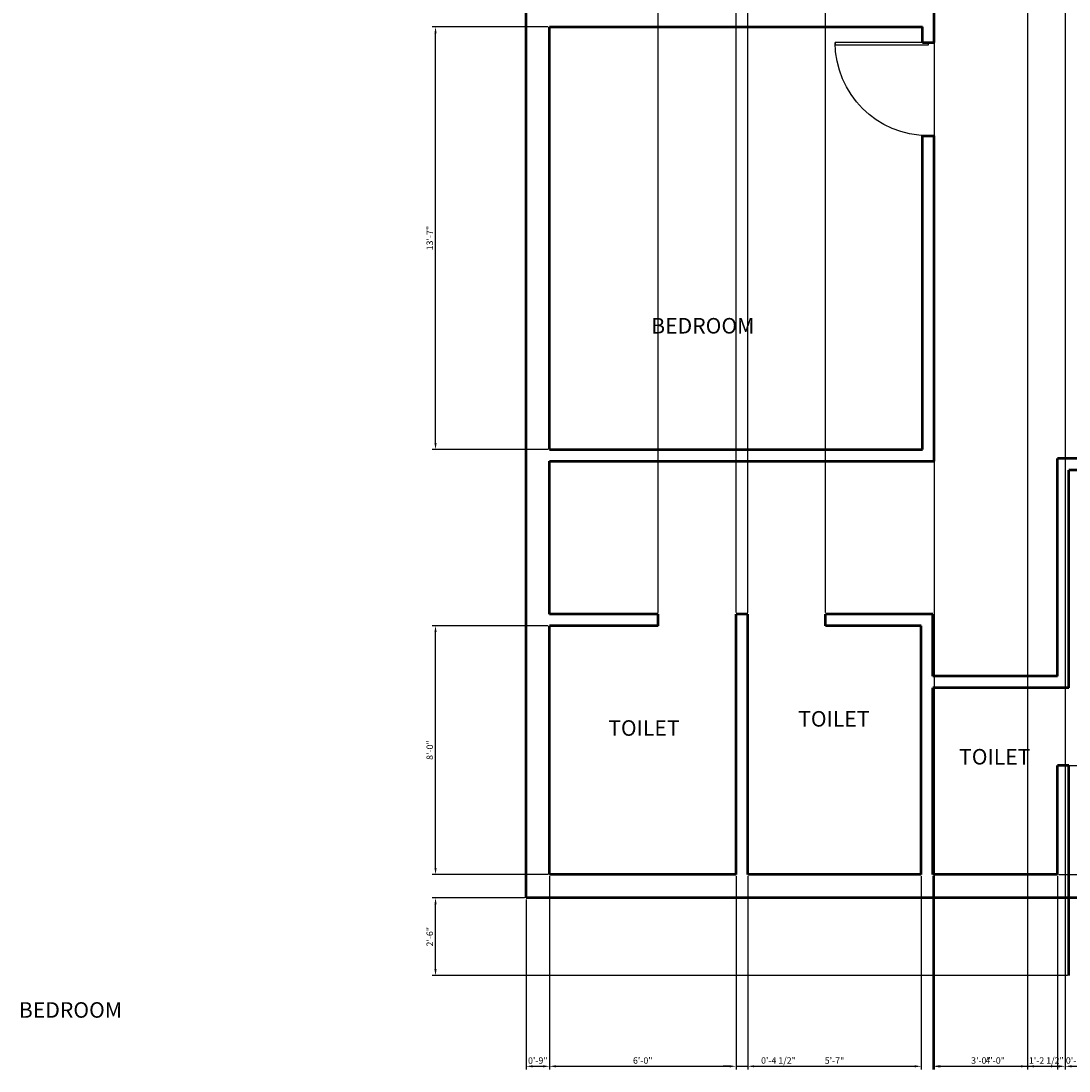
# Model space of a CAD drawing. Units: inches. Extents: x 877 to 2164, y 771 to 1603.
# Tile 1 of 6: x 877 to 1281, y 771 to 1176. Entities that reach past the tile are written whole.
import ezdxf

# ---------------------------------------------------------------- set-up
doc = ezdxf.new("R2010")
doc.units = ezdxf.units.IN
for name, color, linetype, lineweight in [('A-ANNO-DIMS', 2, 'Continuous', 18), ('A-AREA-IDEN', 7, 'Continuous', 25), ('A-DOOR', 5, 'Continuous', 25), ('A-WALL', 7, 'Continuous', 50)]:
    doc.layers.add(name, color=color, linetype=linetype, lineweight=lineweight)
doc.styles.get("Standard").update_dxf_attribs({"font": 'arial.ttf'})
doc.dimstyles.new('ISO-25', dxfattribs={"dimtxt": 2.5, "dimasz": 2.5, "dimexe": 1.25, "dimexo": 0.625, "dimtad": 1, "dimdec": 0, "dimlunit": 4, "dimtxsty": 'Standard', "dimcen": 2.5, "dimadec": 0, "dimazin": 0, "dimtfac": 1, "dimtdec": 0, "dimtmove": 0, "dimatfit": 3, "dimfxl": 1, "dimarcsym": 0})

# ---------------------------------------------------------------- blocks, each defined once
blk = doc.blocks.new('DOOR-SINGLE-36IN')
blk.add_lwpolyline([(0, 0), (0, 1), (36, 1), (36, 0)], close=True)
blk.add_arc((36, 0), 36, 90, 180)
blk = doc.blocks.new('*D16')
at = {"layer": 'A-ANNO-DIMS', "color": 0, "lineweight": -2, "transparency": 16777216}
for p, q in [((1080.27, 1173.62), (1035.67, 1173.62)), ((1036.92, 1013.12), (1036.92, 1171.12)), ((1080.27, 1010.62), (1035.67, 1010.62))]:
    blk.add_line(p, q, dxfattribs=at)
at = {"layer": 'A-ANNO-DIMS', "color": 0, "transparency": 16777216}
for points in [[(1036.5, 1171.12), (1037.34, 1171.12), (1036.92, 1173.62)], [(1036.5, 1013.12), (1037.34, 1013.12), (1036.92, 1010.62)]]:
    blk.add_solid(points, dxfattribs=at)
at = {"layer": 'Defpoints', "color": 0, "transparency": 16777216}
for p in [(1036.92, 1173.62), (1080.89, 1173.62), (1080.89, 1010.62)]:
    blk.add_point(p, dxfattribs=at)
at = {"layer": 'A-ANNO-DIMS', "color": 0, "transparency": 16777216, "insert": (1035.02, 1092.12), "char_height": 2.5, "attachment_point": 5, "rotation": 90}
blk.add_mtext('13\'-7"', dxfattribs=at)
blk = doc.blocks.new('*D24')
at = {"layer": 'A-ANNO-DIMS', "color": 0, "lineweight": -2, "transparency": 16777216}
for p, q in [((1080.89, 846), (1080.89, 771.4)), ((1152.89, 846), (1152.89, 771.4)), ((1083.39, 772.65), (1150.39, 772.65))]:
    blk.add_line(p, q, dxfattribs=at)
at = {"layer": 'A-ANNO-DIMS', "color": 0, "transparency": 16777216}
for points in [[(1083.39, 773.06), (1083.39, 772.23), (1080.89, 772.65)], [(1150.39, 773.06), (1150.39, 772.23), (1152.89, 772.65)]]:
    blk.add_solid(points, dxfattribs=at)
at = {"layer": 'Defpoints', "color": 0, "transparency": 16777216}
for p in [(1080.89, 846.62), (1152.89, 846.62), (1152.89, 772.65)]:
    blk.add_point(p, dxfattribs=at)
at = {"layer": 'A-ANNO-DIMS', "color": 0, "transparency": 16777216, "insert": (1116.89, 774.55), "char_height": 2.5, "attachment_point": 5}
blk.add_mtext('6\'-0"', dxfattribs=at)
blk = doc.blocks.new('*D25')
at = {"layer": 'A-ANNO-DIMS', "color": 0, "lineweight": -2, "transparency": 16777216}
for p, q in [((1157.39, 846), (1157.39, 771.4)), ((1224.39, 846), (1224.39, 771.4)), ((1159.89, 772.65), (1221.89, 772.65))]:
    blk.add_line(p, q, dxfattribs=at)
at = {"layer": 'A-ANNO-DIMS', "color": 0, "transparency": 16777216}
for points in [[(1159.89, 773.06), (1159.89, 772.23), (1157.39, 772.65)], [(1221.89, 773.06), (1221.89, 772.23), (1224.39, 772.65)]]:
    blk.add_solid(points, dxfattribs=at)
at = {"layer": 'Defpoints', "color": 0, "transparency": 16777216}
for p in [(1157.39, 846.62), (1224.39, 846.62), (1224.39, 772.65)]:
    blk.add_point(p, dxfattribs=at)
at = {"layer": 'A-ANNO-DIMS', "color": 0, "transparency": 16777216, "insert": (1190.89, 774.54), "char_height": 2.5, "attachment_point": 5}
blk.add_mtext('5\'-7"', dxfattribs=at)
blk = doc.blocks.new('*D26')
at = {"layer": 'A-ANNO-DIMS', "color": 0, "lineweight": -2, "transparency": 16777216}
for p, q in [((1228.89, 846), (1228.89, 771.4)), ((1276.89, 846), (1276.89, 771.4)), ((1231.39, 772.65), (1274.39, 772.65))]:
    blk.add_line(p, q, dxfattribs=at)
at = {"layer": 'A-ANNO-DIMS', "color": 0, "transparency": 16777216}
for points in [[(1231.39, 773.06), (1231.39, 772.23), (1228.89, 772.65)], [(1274.39, 773.06), (1274.39, 772.23), (1276.89, 772.65)]]:
    blk.add_solid(points, dxfattribs=at)
at = {"layer": 'Defpoints', "color": 0, "transparency": 16777216}
for p in [(1228.89, 846.62), (1276.89, 846.62), (1276.89, 772.65)]:
    blk.add_point(p, dxfattribs=at)
at = {"layer": 'A-ANNO-DIMS', "color": 0, "transparency": 16777216, "insert": (1252.89, 774.55), "char_height": 2.5, "attachment_point": 5}
blk.add_mtext('4\'-0"', dxfattribs=at)
blk = doc.blocks.new('*D28')
at = {"layer": 'A-ANNO-DIMS', "color": 0, "lineweight": -2, "transparency": 16777216}
for p, q in [((1080.27, 942.62), (1035.67, 942.62)), ((1036.92, 849.12), (1036.92, 940.12)), ((1080.27, 846.62), (1035.67, 846.62))]:
    blk.add_line(p, q, dxfattribs=at)
at = {"layer": 'A-ANNO-DIMS', "color": 0, "transparency": 16777216}
for points in [[(1036.5, 940.12), (1037.34, 940.12), (1036.92, 942.62)], [(1036.5, 849.12), (1037.34, 849.12), (1036.92, 846.62)]]:
    blk.add_solid(points, dxfattribs=at)
at = {"layer": 'Defpoints', "color": 0, "transparency": 16777216}
for p in [(1036.92, 942.62), (1080.89, 942.62), (1080.89, 846.62)]:
    blk.add_point(p, dxfattribs=at)
at = {"layer": 'A-ANNO-DIMS', "color": 0, "transparency": 16777216, "insert": (1035.02, 894.62), "char_height": 2.5, "attachment_point": 5, "rotation": 90}
blk.add_mtext('8\'-0"', dxfattribs=at)
blk = doc.blocks.new('*D29')
at = {"layer": 'A-ANNO-DIMS', "color": 0, "lineweight": -2, "transparency": 16777216}
for p, q in [((1277.52, 888.62), (1708.12, 888.62)), ((1706.87, 849.12), (1706.87, 886.12)), ((1277.52, 846.62), (1708.12, 846.62))]:
    blk.add_line(p, q, dxfattribs=at)
at = {"layer": 'A-ANNO-DIMS', "color": 0, "transparency": 16777216}
for points in [[(1706.45, 886.12), (1707.29, 886.12), (1706.87, 888.62)], [(1706.45, 849.12), (1707.29, 849.12), (1706.87, 846.62)]]:
    blk.add_solid(points, dxfattribs=at)
at = {"layer": 'Defpoints', "color": 0, "transparency": 16777216}
for p in [(1276.89, 888.62), (1706.87, 888.62), (1276.89, 846.62)]:
    blk.add_point(p, dxfattribs=at)
at = {"layer": 'A-ANNO-DIMS', "color": 0, "transparency": 16777216, "insert": (1704.97, 867.62), "char_height": 2.5, "attachment_point": 5, "rotation": 90}
blk.add_mtext('3\'-6"', dxfattribs=at)
blk = doc.blocks.new('*D31')
at = {"layer": 'A-ANNO-DIMS', "color": 0, "lineweight": -2, "transparency": 16777216}
for p, q in [((1071.27, 837.62), (1035.67, 837.62)), ((1036.92, 810.12), (1036.92, 835.12)), ((1280.77, 807.62), (1035.67, 807.62))]:
    blk.add_line(p, q, dxfattribs=at)
at = {"layer": 'A-ANNO-DIMS', "color": 0, "transparency": 16777216}
for points in [[(1036.5, 835.12), (1037.34, 835.12), (1036.92, 837.62)], [(1036.5, 810.12), (1037.34, 810.12), (1036.92, 807.62)]]:
    blk.add_solid(points, dxfattribs=at)
at = {"layer": 'Defpoints', "color": 0, "transparency": 16777216}
for p in [(1036.92, 837.62), (1071.89, 837.62), (1281.39, 807.62)]:
    blk.add_point(p, dxfattribs=at)
at = {"layer": 'A-ANNO-DIMS', "color": 0, "transparency": 16777216, "insert": (1035.02, 822.62), "char_height": 2.5, "attachment_point": 5, "rotation": 90}
blk.add_mtext('2\'-6"', dxfattribs=at)
blk = doc.blocks.new('*D32')
at = {"layer": 'A-ANNO-DIMS', "color": 0, "lineweight": -2, "transparency": 16777216}
for p, q in [((1080.89, 846), (1080.89, 771.4)), ((1071.89, 837), (1071.89, 771.4)), ((1074.39, 772.65), (1078.39, 772.65))]:
    blk.add_line(p, q, dxfattribs=at)
at = {"layer": 'A-ANNO-DIMS', "color": 0, "transparency": 16777216}
for points in [[(1074.39, 773.06), (1074.39, 772.23), (1071.89, 772.65)], [(1078.39, 773.06), (1078.39, 772.23), (1080.89, 772.65)]]:
    blk.add_solid(points, dxfattribs=at)
at = {"layer": 'Defpoints', "color": 0, "transparency": 16777216}
for p in [(1080.89, 846.62), (1071.89, 837.62), (1080.89, 772.65)]:
    blk.add_point(p, dxfattribs=at)
at = {"layer": 'A-ANNO-DIMS', "color": 0, "transparency": 16777216, "insert": (1076.39, 774.55), "char_height": 2.5, "attachment_point": 5}
blk.add_mtext('0\'-9"', dxfattribs=at)
blk = doc.blocks.new('*D33')
at = {"layer": 'A-ANNO-DIMS', "color": 0, "lineweight": -2, "transparency": 16777216}
for p, q in [((1152.89, 846), (1152.89, 771.4)), ((1157.39, 846), (1157.39, 771.4)), ((1150.39, 772.65), (1147.89, 772.65)), ((1152.89, 772.65), (1157.39, 772.65)), ((1159.89, 772.65), (1176.12, 772.65))]:
    blk.add_line(p, q, dxfattribs=at)
at = {"layer": 'A-ANNO-DIMS', "color": 0, "transparency": 16777216}
for points in [[(1150.39, 773.06), (1150.39, 772.23), (1152.89, 772.65)], [(1159.89, 773.06), (1159.89, 772.23), (1157.39, 772.65)]]:
    blk.add_solid(points, dxfattribs=at)
at = {"layer": 'Defpoints', "color": 0, "transparency": 16777216}
for p in [(1152.89, 846.62), (1157.39, 846.62), (1157.39, 772.65)]:
    blk.add_point(p, dxfattribs=at)
at = {"layer": 'A-ANNO-DIMS', "color": 0, "transparency": 16777216, "insert": (1169.26, 774.56), "char_height": 2.5, "attachment_point": 5}
blk.add_mtext('0\'-4 1/2"', dxfattribs=at)
blk = doc.blocks.new('*D34')
at = {"layer": 'A-ANNO-DIMS', "color": 0, "lineweight": -2, "transparency": 16777216}
for p, q in [((1122.89, 947.75), (1122.89, 1533.85)), ((1125.39, 1532.6), (1150.39, 1532.6)), ((1152.89, 947.75), (1152.89, 1533.85))]:
    blk.add_line(p, q, dxfattribs=at)
at = {"layer": 'A-ANNO-DIMS', "color": 0, "transparency": 16777216}
for points in [[(1125.39, 1533.01), (1125.39, 1532.18), (1122.89, 1532.6)], [(1150.39, 1533.01), (1150.39, 1532.18), (1152.89, 1532.6)]]:
    blk.add_solid(points, dxfattribs=at)
at = {"layer": 'Defpoints', "color": 0, "transparency": 16777216}
for p in [(1152.89, 1532.6), (1122.89, 947.12), (1152.89, 947.12)]:
    blk.add_point(p, dxfattribs=at)
at = {"layer": 'A-ANNO-DIMS', "color": 0, "transparency": 16777216, "insert": (1137.89, 1534.5), "char_height": 2.5, "attachment_point": 5}
blk.add_mtext('2\'-6"', dxfattribs=at)
blk = doc.blocks.new('*D35')
at = {"layer": 'A-ANNO-DIMS', "color": 0, "lineweight": -2, "transparency": 16777216}
for p, q in [((1157.39, 947.75), (1157.39, 1533.85)), ((1159.89, 1532.6), (1184.89, 1532.6)), ((1187.39, 947.75), (1187.39, 1533.85))]:
    blk.add_line(p, q, dxfattribs=at)
at = {"layer": 'A-ANNO-DIMS', "color": 0, "transparency": 16777216}
for points in [[(1159.89, 1533.01), (1159.89, 1532.18), (1157.39, 1532.6)], [(1184.89, 1533.01), (1184.89, 1532.18), (1187.39, 1532.6)]]:
    blk.add_solid(points, dxfattribs=at)
at = {"layer": 'Defpoints', "color": 0, "transparency": 16777216}
for p in [(1187.39, 1532.6), (1157.39, 947.12), (1187.39, 947.12)]:
    blk.add_point(p, dxfattribs=at)
at = {"layer": 'A-ANNO-DIMS', "color": 0, "transparency": 16777216, "insert": (1172.39, 1534.5), "char_height": 2.5, "attachment_point": 5}
blk.add_mtext('2\'-6"', dxfattribs=at)
blk = doc.blocks.new('*D37')
at = {"layer": 'A-ANNO-DIMS', "color": 0, "lineweight": -2, "transparency": 16777216}
for p, q in [((1229.39, 1392), (1229.39, 771.4)), ((1265.39, 1392), (1265.39, 771.4)), ((1231.89, 772.65), (1262.89, 772.65))]:
    blk.add_line(p, q, dxfattribs=at)
at = {"layer": 'A-ANNO-DIMS', "color": 0, "transparency": 16777216}
for points in [[(1231.89, 773.06), (1231.89, 772.23), (1229.39, 772.65)], [(1262.89, 773.06), (1262.89, 772.23), (1265.39, 772.65)]]:
    blk.add_solid(points, dxfattribs=at)
at = {"layer": 'Defpoints', "color": 0, "transparency": 16777216}
for p in [(1229.39, 1392.62), (1265.39, 1392.62), (1265.39, 772.65)]:
    blk.add_point(p, dxfattribs=at)
at = {"layer": 'A-ANNO-DIMS', "color": 0, "transparency": 16777216, "insert": (1247.39, 774.55), "char_height": 2.5, "attachment_point": 5}
blk.add_mtext('3\'-0"', dxfattribs=at)
blk = doc.blocks.new('*D43')
at = {"layer": 'A-ANNO-DIMS', "color": 0, "lineweight": -2, "transparency": 16777216}
for p, q in [((1279.89, 1452), (1279.89, 771.4)), ((1265.39, 1442), (1265.39, 771.4)), ((1267.89, 772.65), (1277.39, 772.65))]:
    blk.add_line(p, q, dxfattribs=at)
at = {"layer": 'A-ANNO-DIMS', "color": 0, "transparency": 16777216}
for points in [[(1267.89, 773.06), (1267.89, 772.23), (1265.39, 772.65)], [(1277.39, 773.06), (1277.39, 772.23), (1279.89, 772.65)]]:
    blk.add_solid(points, dxfattribs=at)
at = {"layer": 'Defpoints', "color": 0, "transparency": 16777216}
for p in [(1279.89, 1452.62), (1265.39, 1442.62), (1279.89, 772.65)]:
    blk.add_point(p, dxfattribs=at)
at = {"layer": 'A-ANNO-DIMS', "color": 0, "transparency": 16777216, "insert": (1272.64, 774.56), "char_height": 2.5, "attachment_point": 5}
blk.add_mtext('1\'-2 1/2"', dxfattribs=at)
blk = doc.blocks.new('*D44')
at = {"layer": 'A-ANNO-DIMS', "color": 0, "lineweight": -2, "transparency": 16777216}
for p, q in [((1279.89, 1452), (1279.89, 771.4)), ((1289.89, 1452), (1289.89, 771.4)), ((1282.39, 772.65), (1287.39, 772.65))]:
    blk.add_line(p, q, dxfattribs=at)
at = {"layer": 'A-ANNO-DIMS', "color": 0, "transparency": 16777216}
for points in [[(1282.39, 773.06), (1282.39, 772.23), (1279.89, 772.65)], [(1287.39, 773.06), (1287.39, 772.23), (1289.89, 772.65)]]:
    blk.add_solid(points, dxfattribs=at)
at = {"layer": 'Defpoints', "color": 0, "transparency": 16777216}
for p in [(1279.89, 1452.62), (1289.89, 1452.62), (1289.89, 772.65)]:
    blk.add_point(p, dxfattribs=at)
at = {"layer": 'A-ANNO-DIMS', "color": 0, "transparency": 16777216, "insert": (1284.89, 774.55), "char_height": 2.5, "attachment_point": 5}
blk.add_mtext('0\'-10"', dxfattribs=at)

msp = doc.modelspace()

# ---------------------------------------------------------------- linework, layer by layer
at = {"layer": 'A-WALL'}
for p, q in [((1071.89, 837.62), (1071.89, 1497.62)), ((1229.39, 1167.62), (1229.39, 1298.12)), ((1080.89, 1173.62), (1224.89, 1173.62)), ((1080.89, 1010.62), (1080.89, 1173.62)), ((1224.89, 1167.62), (1224.89, 1173.62)), ((1224.89, 1167.62), (1229.39, 1167.62)), ((1224.89, 1010.62), (1224.89, 1131.62)), ((1224.89, 1131.62), (1229.39, 1131.62)), ((1229.39, 1006.12), (1229.39, 1131.62)), ((1080.89, 1010.62), (1224.89, 1010.62)), ((1080.89, 1006.12), (1229.39, 1006.12)), ((1080.89, 947.12), (1080.89, 1006.12)), ((1276.89, 923.12), (1276.89, 1007.12)), ((1373.89, 1007.12), (1276.89, 1007.12)), ((1281.39, 918.62), (1281.39, 1002.62)), ((1373.89, 1002.62), (1281.39, 1002.62)), ((1122.89, 947.12), (1080.89, 947.12)), ((1122.89, 942.62), (1122.89, 947.12)), ((1152.89, 846.62), (1152.89, 947.12)), ((1157.39, 947.12), (1152.89, 947.12)), ((1157.39, 846.62), (1157.39, 947.12)), ((1228.89, 947.12), (1187.39, 947.12)), ((1187.39, 942.62), (1187.39, 947.12)), ((1228.89, 923.12), (1228.89, 947.12)), ((1080.89, 846.62), (1080.89, 942.62)), ((1122.89, 942.62), (1080.89, 942.62)), ((1224.39, 942.62), (1187.39, 942.62)), ((1224.39, 846.62), (1224.39, 942.62)), ((1276.89, 923.12), (1228.89, 923.12)), ((1228.89, 846.62), (1228.89, 918.62)), ((1281.39, 918.62), (1228.89, 918.62)), ((1276.89, 846.62), (1276.89, 888.62)), ((1281.39, 888.62), (1276.89, 888.62)), ((1281.39, 807.62), (1281.39, 888.62)), ((1152.89, 846.62), (1080.89, 846.62)), ((1224.39, 846.62), (1157.39, 846.62)), ((1276.89, 846.62), (1228.89, 846.62)), ((1671.89, 837.62), (1071.89, 837.62))]:
    msp.add_line(p, q, dxfattribs=at)

# ---------------------------------------------------------------- block references
at = {"layer": 'A-DOOR', "extrusion": (0, 0, -1), "zscale": -1, "rotation": 180}
msp.add_blockref('DOOR-SINGLE-36IN', (-1191.15, 1167.62), dxfattribs=at)

# ---------------------------------------------------------------- texts
at = {"layer": 'A-AREA-IDEN', "char_height": 6, "attachment_point": 1}
for s, width, insert in [('BEDROOM', 54.8109, (1120.14, 1061.31)), ('TOILET', 34.9534, (1176.87, 909.68)), ('TOILET', 34.9534, (1103.56, 906.14)), ('TOILET', 34.9534, (1238.97, 895.05)), ('BEDROOM', 54.8109, (876.12, 797.38))]:
    msp.add_mtext_dynamic_manual_height_columns(s, width=width, gutter_width=12.5, heights=[0], dxfattribs=dict(at, insert=insert))

# ---------------------------------------------------------------- dimensions: what is measured, and where the dimension line sits
at = {"layer": 'A-ANNO-DIMS'}
for base, p1, p2, picture, middle in [((1152.89, 1532.6), (1122.89, 947.12), (1152.89, 947.12), '*D34', (1137.89, 1534.5)), ((1187.39, 1532.6), (1157.39, 947.12), (1187.39, 947.12), '*D35', (1172.39, 1534.5)), ((1279.89, 772.65), (1265.39, 1442.62), (1279.89, 1452.62), '*D43', (1272.64, 774.56)), ((1289.89, 772.65), (1279.89, 1452.62), (1289.89, 1452.62), '*D44', (1284.89, 774.55)), ((1265.39, 772.65), (1229.39, 1392.62), (1265.39, 1392.62), '*D37', (1247.39, 774.55)), ((1080.89, 772.65), (1071.89, 837.62), (1080.89, 846.62), '*D32', (1076.39, 774.55)), ((1152.89, 772.65), (1080.89, 846.62), (1152.89, 846.62), '*D24', (1116.89, 774.55)), ((1157.39, 772.65), (1152.89, 846.62), (1157.39, 846.62), '*D33', (1169.26, 774.56)), ((1224.39, 772.65), (1157.39, 846.62), (1224.39, 846.62), '*D25', (1190.89, 774.54)), ((1276.89, 772.65), (1228.89, 846.62), (1276.89, 846.62), '*D26', (1252.89, 774.55))]:
    dim = msp.add_linear_dim(base=base, p1=p1, p2=p2, dimstyle='ISO-25', override={"dimdec": 1, "dimlfac": 1, "dimrnd": 0, "dimzin": 1, "dimdsep": 46, "dimlunit": 4, "dimfrac": 2}, dxfattribs=at)
    dim.commit()
    dim.dimension.update_dxf_attribs({"geometry": picture, "text_midpoint": middle})
for base, p1, p2, picture, middle in [((1036.92, 1173.62), (1080.89, 1010.62), (1080.89, 1173.62), '*D16', (1035.02, 1092.12)), ((1036.92, 942.62), (1080.89, 846.62), (1080.89, 942.62), '*D28', (1035.02, 894.62)), ((1706.87, 888.62), (1276.89, 846.62), (1276.89, 888.62), '*D29', (1704.97, 867.62)), ((1036.92, 837.62), (1281.39, 807.62), (1071.89, 837.62), '*D31', (1035.02, 822.62))]:
    dim = msp.add_linear_dim(base=base, p1=p1, p2=p2, angle=90, dimstyle='ISO-25', override={"dimdec": 1, "dimlfac": 1, "dimrnd": 0, "dimzin": 1, "dimdsep": 46, "dimlunit": 4, "dimfrac": 2}, dxfattribs=at)
    dim.commit()
    dim.dimension.update_dxf_attribs({"geometry": picture, "text_midpoint": middle})

doc.saveas('drawing.dxf')
